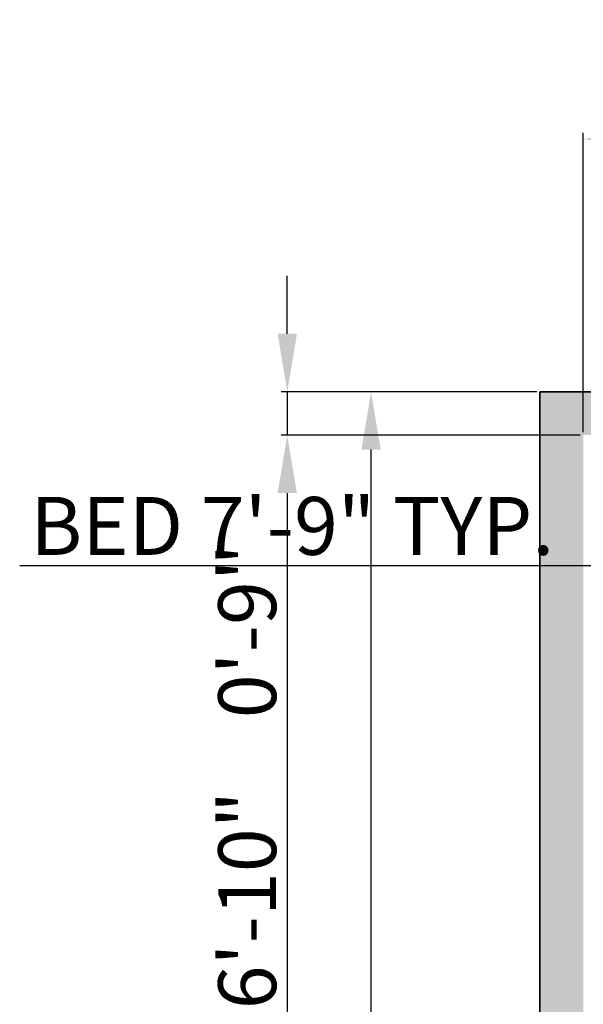
# Model space of a CAD drawing. Units: inches. Extents: x 2083 to 3317, y 1141 to 2115.
# Tile 94 of 256: x 2119 to 2236, y 1894 to 2098. Entities that reach past the tile are written whole.
import ezdxf

# ---------------------------------------------------------------- set-up
doc = ezdxf.new("R2010")
doc.units = ezdxf.units.IN
doc.layers.add('A-ANNO-DIMS', color=2, linetype='Continuous', lineweight=18)
doc.layers.add('A-WALL', color=7, linetype='Continuous', lineweight=35)
doc.layers.add('A-WALL-PATT', color=251, linetype='Continuous', lineweight=13, true_color=0x636466)
doc.styles.get("Standard").update_dxf_attribs({"font": 'arial.ttf'})
doc.dimstyles.new('ISO-25', dxfattribs={"dimtxt": 12, "dimasz": 12, "dimexe": 1.25, "dimexo": 0.625, "dimtad": 1, "dimlunit": 3, "dimtxsty": 'Standard', "dimcen": 2.5, "dimadec": 0, "dimazin": 0, "dimtfac": 1, "dimtmove": 0, "dimatfit": 3, "dimfxl": 1, "dimarcsym": 0})

# ---------------------------------------------------------------- blocks, each defined once
blk = doc.blocks.new('*D14')
at = {"layer": 'A-ANNO-DIMS', "color": 0, "lineweight": -2, "transparency": 16777216}
for p, q in [((2226.33, 2020.76), (2190.73, 2020.76)), ((2191.98, 1714.76), (2191.98, 2008.76)), ((2226.33, 1702.76), (2190.73, 1702.76))]:
    blk.add_line(p, q, dxfattribs=at)
at = {"layer": 'A-ANNO-DIMS', "color": 0, "transparency": 16777216}
for points in [[(2189.98, 2008.76), (2193.98, 2008.76), (2191.98, 2020.76)], [(2189.98, 1714.76), (2193.98, 1714.76), (2191.98, 1702.76)]]:
    blk.add_solid(points, dxfattribs=at)
at = {"layer": 'Defpoints', "color": 0, "transparency": 16777216}
for p in [(2191.98, 2020.76), (2226.96, 2020.76), (2226.96, 1702.76)]:
    blk.add_point(p, dxfattribs=at)
at = {"layer": 'A-ANNO-DIMS', "color": 0, "transparency": 16777216, "insert": (2185.22, 1861.76), "char_height": 12, "attachment_point": 5, "rotation": 90}
blk.add_mtext('26\'-6"', dxfattribs=at)
blk = doc.blocks.new('*D20')
at = {"layer": 'A-ANNO-DIMS', "color": 0, "lineweight": -2, "transparency": 16777216}
for p, q in [((2244.15, 1971.32), (2244.15, 1985.9)), ((2337.22, 1971.32), (2337.22, 1985.9)), ((2244.15, 1984.65), (2119.16, 1984.65)), ((2325.22, 1984.65), (2256.15, 1984.65))]:
    blk.add_line(p, q, dxfattribs=at)
at = {"layer": 'A-ANNO-DIMS', "color": 0, "transparency": 16777216}
for points in [[(2256.15, 1986.65), (2256.15, 1982.65), (2244.15, 1984.65)], [(2325.22, 1986.65), (2325.22, 1982.65), (2337.22, 1984.65)]]:
    blk.add_solid(points, dxfattribs=at)
at = {"layer": 'Defpoints', "color": 0, "transparency": 16777216}
for p in [(2244.15, 1984.65), (2244.15, 1970.69), (2337.22, 1970.69)]:
    blk.add_point(p, dxfattribs=at)
at = {"layer": 'A-ANNO-DIMS', "color": 0, "transparency": 16777216, "insert": (2175.65, 1991.4), "char_height": 12, "attachment_point": 5}
blk.add_mtext('BED 7\'-9" TYP.', dxfattribs=at)
blk = doc.blocks.new('*D36')
at = {"layer": 'A-ANNO-DIMS', "color": 0, "lineweight": -2, "transparency": 16777216}
for p, q in [((2235.96, 2012.39), (2235.96, 2074.36)), ((2247.96, 2073.11), (2459.46, 2073.11)), ((2471.46, 2012.39), (2471.46, 2074.36))]:
    blk.add_line(p, q, dxfattribs=at)
at = {"layer": 'A-ANNO-DIMS', "color": 0, "transparency": 16777216}
for points in [[(2247.96, 2075.11), (2247.96, 2071.11), (2235.96, 2073.11)], [(2459.46, 2075.11), (2459.46, 2071.11), (2471.46, 2073.11)]]:
    blk.add_solid(points, dxfattribs=at)
at = {"layer": 'Defpoints', "color": 0, "transparency": 16777216}
for p in [(2471.46, 2073.11), (2235.96, 2011.76), (2471.46, 2011.76)]:
    blk.add_point(p, dxfattribs=at)
at = {"layer": 'A-ANNO-DIMS', "color": 0, "transparency": 16777216, "insert": (2353.71, 2079.94), "char_height": 12, "attachment_point": 5}
blk.add_mtext('19\'-7 1/2"', dxfattribs=at)
blk = doc.blocks.new('*D39')
at = {"layer": 'A-ANNO-DIMS', "color": 0, "lineweight": -2, "transparency": 16777216}
for p, q in [((2235.33, 2011.76), (2173.36, 2011.76)), ((2174.61, 1999.76), (2174.61, 1822.01)), ((2235.33, 1810.01), (2173.36, 1810.01))]:
    blk.add_line(p, q, dxfattribs=at)
at = {"layer": 'A-ANNO-DIMS', "color": 0, "transparency": 16777216}
for points in [[(2172.61, 1999.76), (2176.61, 1999.76), (2174.61, 2011.76)], [(2172.61, 1822.01), (2176.61, 1822.01), (2174.61, 1810.01)]]:
    blk.add_solid(points, dxfattribs=at)
at = {"layer": 'Defpoints', "color": 0, "transparency": 16777216}
for p in [(2235.96, 2011.76), (2174.61, 1810.01), (2235.96, 1810.01)]:
    blk.add_point(p, dxfattribs=at)
at = {"layer": 'A-ANNO-DIMS', "color": 0, "transparency": 16777216, "insert": (2167.86, 1910.89), "char_height": 12, "attachment_point": 5, "rotation": 90}
blk.add_mtext('16\'-10"', dxfattribs=at)
blk = doc.blocks.new('*D49')
at = {"layer": 'A-ANNO-DIMS', "color": 0, "lineweight": -2, "transparency": 16777216}
for p, q in [((2174.61, 2032.76), (2174.61, 2044.76)), ((2226.33, 2020.76), (2173.36, 2020.76)), ((2174.61, 2020.76), (2174.61, 2011.76)), ((2235.33, 2011.76), (2173.36, 2011.76)), ((2174.61, 1999.76), (2174.61, 1954.61))]:
    blk.add_line(p, q, dxfattribs=at)
at = {"layer": 'A-ANNO-DIMS', "color": 0, "transparency": 16777216}
for points in [[(2172.61, 2032.76), (2176.61, 2032.76), (2174.61, 2020.76)], [(2172.61, 1999.76), (2176.61, 1999.76), (2174.61, 2011.76)]]:
    blk.add_solid(points, dxfattribs=at)
at = {"layer": 'Defpoints', "color": 0, "transparency": 16777216}
for p in [(2226.96, 2020.76), (2174.61, 2011.76), (2235.96, 2011.76)]:
    blk.add_point(p, dxfattribs=at)
at = {"layer": 'A-ANNO-DIMS', "color": 0, "transparency": 16777216, "insert": (2167.86, 1971.19), "char_height": 12, "attachment_point": 5, "rotation": 90}
blk.add_mtext('0\'-9"', dxfattribs=at)

msp = doc.modelspace()

# ---------------------------------------------------------------- hatches: boundary and pattern name
at = {"layer": 'A-WALL-PATT'}
h = msp.add_hatch(color=256, dxfattribs=at)
h.dxf.hatch_style = 1
h.paths.add_polyline_path([(3126.96, 2020.761), (2748.96, 2020.761), (2604.96, 2020.761), (2226.96, 2020.761), (2226.96, 1702.761), (2466.96, 1702.761), (2466.96, 1582.761), (2418.96, 1582.761), (2418.96, 1477.761), (2226.96, 1477.761), (2226.96, 1263.261), (2544.96, 1263.261), (2544.96, 1411.761), (2604.96, 1411.761), (2685.96, 1411.761), (2685.96, 1420.761), (2604.96, 1420.761), (2604.96, 1573.761), (2604.96, 1702.761), (2604.96, 2011.761), (2748.96, 2011.761), (2748.96, 1702.761), (2862.96, 1702.761), (2862.96, 1621.761), (2871.96, 1621.761), (2871.96, 1702.761), (2883.96, 1702.761), (2883.96, 1706.939, -0.0264593), (2883.96, 1711.761), (2757.96, 1711.761), (2757.96, 1807.761), (2787.96, 1807.761), (2787.96, 1812.261), (2757.96, 1812.261), (2757.96, 2011.761), (2877.96, 2011.761), (2877.96, 1812.261), (2847.96, 1812.261), (2847.96, 1807.761), (2889.836, 1807.761), (2889.836, 1812.261), (2882.46, 1812.261), (2882.46, 2011.761), (3117.96, 2011.761), (3117.96, 1812.261), (2937.836, 1812.261), (2937.836, 1807.761), (2995.71, 1807.761), (2995.71, 1796.118), (3000.21, 1796.118), (3000.21, 1807.761), (3117.96, 1807.761), (3117.96, 1711.761), (3000.21, 1711.761), (3000.21, 1760.118), (2998.573, 1760.118, -0.020711), (2995.71, 1760.118), (2995.71, 1711.761), (2931.96, 1711.761), (2931.96, 1702.761), (3126.96, 1702.761)])
h.paths.add_polyline_path([(2471.46, 2011.761), (2471.46, 1810.011), (2462.717, 1810.011), (2462.717, 1805.511), (2505.96, 1805.511), (2505.96, 1810.011), (2475.96, 1810.011), (2475.96, 2011.761), (2595.96, 2011.761), (2595.96, 1810.011), (2565.96, 1810.011), (2565.96, 1805.511), (2595.96, 1805.511), (2595.96, 1711.761), (2235.96, 1711.761), (2235.96, 1805.511), (2353.71, 1805.511), (2353.71, 1796.054), (2358.21, 1796.054), (2358.21, 1805.511), (2414.717, 1805.511), (2414.717, 1810.011), (2235.96, 1810.011), (2235.96, 2011.761)], flags=16)
h.paths.add_polyline_path([(2270.205, 1994.61), (2270.205, 1970.61), (2246.205, 1970.61), (2246.205, 1994.61)], flags=0)
edge = h.paths.add_edge_path(flags=0)
edge.add_ellipse((2332.027, 1899.798), major_axis=(-3.043, 3.043), ratio=0.1682525, start_angle=-161.33217, end_angle=-156.30711, ccw=False)
edge.add_ellipse((2333.082, 1898.744), major_axis=(-1.055, 1.055), ratio=0.4535321, start_angle=-123.37102, end_angle=-94.15911)
edge = h.paths.add_edge_path(flags=0)
edge.add_ellipse((2332.027, 1968.876), major_axis=(3.043, 3.043), ratio=0.1682525, start_angle=18.66783, end_angle=23.69289)
edge.add_spline(control_points=[(2332.926, 1970.691), (2332.227, 1970.336), (2330.894, 1969.659), (2328.413, 1970.932), (2327.204, 1967.749), (2324.71, 1969.956), (2322.533, 1967.012), (2320.013, 1971.296), (2317.68, 1968.158), (2316.041, 1967.102), (2315.427, 1966.81)], knot_values=[0, 0, 0, 0, 2.2670587, 4.3245589, 6.6855835, 8.8786411, 11.121502, 14.300359, 17.7552837, 19.732645, 19.732645, 19.732645, 19.732645], degree=3, periodic=0)
edge.add_ellipse((2332.027, 1968.876), major_axis=(3.043, 3.043), ratio=0.1682525, start_angle=18.66783, end_angle=23.69289, ccw=False)
edge.add_ellipse((2333.082, 1969.931), major_axis=(1.055, 1.055), ratio=0.4535321, start_angle=56.62898, end_angle=85.84089, ccw=False)
edge = h.paths.add_edge_path(flags=0)
edge.add_spline(control_points=[(2296.428, 1967.988), (2293.628, 1965.336), (2287.704, 1959.727), (2299.744, 1949.996), (2294.533, 1935.669), (2290.573, 1920.604), (2293.394, 1909.974), (2296.185, 1904.967)], knot_values=[0.0991853, 0.0991853, 0.0991853, 0.0991853, 0.3453009, 0.6198217, 0.9826526, 1.3860932, 1.8105546, 1.8105546, 1.8105546, 1.8105546], degree=3, periodic=0)
edge.add_spline(control_points=[(2296.185, 1904.967), (2297.384, 1902.619), (2298.001, 1901.949), (2298.553, 1901.468)], knot_values=[0.0062457, 0.0062457, 0.0062457, 0.0062457, 0.0554759, 0.0554759, 0.0554759, 0.0554759], degree=3, periodic=0)
edge.add_spline(control_points=[(2298.553, 1901.468), (2297.259, 1900.923), (2295.225, 1900.232), (2293.06, 1900.614), (2292.101, 1900.788), (2292.09, 1900.791)], knot_values=[0.3128349, 0.3128349, 0.3128349, 0.3128349, 0.4017797, 0.4749867, 0.4759027, 0.4759027, 0.4759027, 0.4759027], degree=3, periodic=0)
edge.add_arc((2292.794, 1904.664), 3.937, 215.4209, 259.69818, ccw=False)
edge.add_spline(control_points=[(2289.585, 1902.382), (2289.477, 1902.535), (2289.368, 1902.688), (2289.261, 1902.841)], knot_values=[0.1028719, 0.1028719, 0.1028719, 0.1028719, 0.1168958, 0.1168958, 0.1168958, 0.1168958], degree=3, periodic=0)
edge.add_spline(control_points=[(2289.261, 1902.841), (2288.687, 1902.55), (2287.64, 1902.02), (2285.881, 1901.874), (2283.853, 1901.504), (2281.72, 1899.711), (2278.467, 1899.493), (2276.157, 1901.883), (2272.259, 1899.804), (2267.778, 1901.843), (2262.244, 1900.184), (2257.415, 1901.782), (2254.318, 1900.726), (2253.178, 1900.337)], knot_values=[0, 0, 0, 0, 1.9079767, 3.4771759, 5.261074, 7.9728515, 11.6802485, 13.7179214, 16.9395917, 22.789562, 27.5025027, 33.5952153, 37.1456181, 37.1456181, 37.1456181, 37.1456181], degree=3, periodic=0)
edge.add_line((2253.178, 1900.337), (2250.244, 1902.841))
edge.add_line((2250.244, 1902.841), (2250.244, 1965.833))
edge.add_line((2250.244, 1965.833), (2253.178, 1968.337))
edge.add_spline(control_points=[(2253.178, 1968.337), (2254.318, 1967.948), (2257.415, 1966.892), (2262.244, 1968.49), (2267.778, 1966.831), (2271.527, 1968.537), (2273.876, 1967.828), (2274.207, 1967.728)], knot_values=[0, 0, 0, 0, 0.0901802, 0.2449351, 0.3646438, 0.5132331, 0.5378548, 0.5378548, 0.5378548, 0.5378548], degree=3, periodic=0)
edge.add_arc((2274.353, 1963.793), 3.937, 72.05113, 92.12795, ccw=False)
edge.add_arc((2281.297, 1985.23), 18.596, 252.05113, 288.56572)
edge.add_arc((2292.317, 1956.029), 12.646, 71.02679, 113.77822, ccw=False)
edge = h.paths.add_edge_path(flags=0)
edge.add_spline(control_points=[(2274.899, 1951.856), (2275.066, 1951.617), (2275.233, 1951.377), (2275.398, 1951.136)], knot_values=[1.4099157, 1.4099157, 1.4099157, 1.4099157, 1.4315903, 1.4315903, 1.4315903, 1.4315903], degree=3, periodic=0)
edge.add_spline(control_points=[(2275.398, 1951.136), (2275.792, 1950.562), (2276.179, 1949.984), (2276.546, 1949.397)], knot_values=[1.3582378, 1.3582378, 1.3582378, 1.3582378, 1.4099157, 1.4099157, 1.4099157, 1.4099157], degree=3, periodic=0)
edge.add_line((2276.546, 1949.397), (2277.437, 1947.862))
edge.add_spline(control_points=[(2277.437, 1947.862), (2276.304, 1945.673), (2274.64, 1942.427), (2274.632, 1938.094), (2272.799, 1930.852), (2274.356, 1943.897), (2275.948, 1947.923), (2276.546, 1949.397)], knot_values=[0.0056315, 0.0056315, 0.0056315, 0.0056315, 0.1860139, 0.2660015, 0.3570872, 0.5963902, 0.7397317, 0.7397317, 0.7397317, 0.7397317], degree=3, periodic=0)
edge.add_spline(control_points=[(2276.546, 1949.397), (2276.179, 1949.984), (2275.792, 1950.562), (2275.398, 1951.136)], knot_values=[1.3582378, 1.3582378, 1.3582378, 1.3582378, 1.4099157, 1.4099157, 1.4099157, 1.4099157], degree=3, periodic=0)
edge.add_spline(control_points=[(2275.398, 1951.136), (2274.943, 1950.08), (2274.208, 1948.025), (2273.935, 1944.851), (2272.469, 1937.627), (2273.466, 1945.696), (2274.701, 1951.059), (2274.899, 1951.856)], knot_values=[0.1043639, 0.1043639, 0.1043639, 0.1043639, 0.1896363, 0.2696239, 0.3607096, 0.6000126, 0.6446217, 0.6446217, 0.6446217, 0.6446217], degree=3, periodic=0)
h.paths.add_polyline_path([(2269.168, 1963.128, -0.3575267), (2268.171, 1960.976, -0.0925607), (2268.171, 1939.436, -0.3575267), (2269.168, 1937.285, -0.3575267), (2267.016, 1938.282, -0.1647847), (2254.686, 1938.282, -0.3575267), (2252.534, 1937.285, -0.3575267), (2253.531, 1939.436, -0.0925607), (2253.531, 1960.976, -0.3575267), (2252.534, 1963.128, -0.3575267), (2254.686, 1962.131, -0.1647847), (2267.016, 1962.131, -0.3575267)], flags=0)
h.paths.add_polyline_path([(2248.874, 1967.802), (2248.874, 1957.028), (2249.458, 1957.028), (2249.458, 1911.647), (2248.874, 1911.647), (2248.874, 1900.873), (2246.512, 1900.873, 0.1973271), (2244.15, 1902.457), (2244.15, 1966.218, 0.1973271), (2246.512, 1967.802)], flags=0)
h.paths.add_polyline_path([(2269.168, 1931.389, -0.3575267), (2268.171, 1929.238, -0.0925607), (2268.171, 1907.698, -0.3575267), (2269.168, 1905.547, -0.3575267), (2267.016, 1906.544, -0.1647847), (2254.686, 1906.544, -0.3575267), (2252.534, 1905.547, -0.3575267), (2253.531, 1907.698, -0.0925607), (2253.531, 1929.238, -0.3575267), (2252.534, 1931.389, -0.3575267), (2254.686, 1930.392, -0.1647847), (2267.016, 1930.392, -0.3575267)], flags=0)
edge = h.paths.add_edge_path(flags=0)
edge.add_spline(control_points=[(2276.197, 1906.724), (2276.168, 1909.029), (2276.114, 1913.372), (2270.598, 1924.925), (2273.905, 1919.013), (2275.922, 1916.262), (2275.475, 1912.402), (2277.258, 1910.381), (2276.696, 1908.225), (2276.646, 1906.813), (2276.618, 1906.008)], knot_values=[0, 0, 0, 0, 8.6102597, 16.2212739, 18.8430575, 23.8048978, 27.4408283, 29.3561016, 31.2034776, 33.6506866, 33.6506866, 33.6506866, 33.6506866], degree=3, periodic=0)
edge.add_spline(control_points=[(2276.618, 1906.008), (2276.623, 1905.624), (2276.498, 1904.629), (2275.442, 1903.855), (2274.937, 1903.08), (2274.859, 1902.841)], knot_values=[0.1564884, 0.1564884, 0.1564884, 0.1564884, 0.1843975, 0.2313765, 0.2505985, 0.2505985, 0.2505985, 0.2505985], degree=3, periodic=0)
edge.add_line((2274.859, 1902.841), (2276.506, 1902.841))
edge.add_spline(control_points=[(2276.506, 1902.841), (2276.788, 1903.085), (2277.665, 1904.125), (2278.25, 1904.341), (2277.654, 1908.527), (2278.156, 1906.228), (2278.1, 1905.286), (2278.847, 1904.069), (2277.857, 1903.415), (2277.874, 1902.991), (2277.904, 1902.841)], knot_values=[0.0595743, 0.0595743, 0.0595743, 0.0595743, 0.0807529, 0.1037415, 0.1697201, 0.1760361, 0.2071372, 0.2404744, 0.2623409, 0.2736605, 0.2736605, 0.2736605, 0.2736605], degree=3, periodic=0)
edge.add_line((2277.904, 1902.841), (2280.03, 1902.841))
edge.add_spline(control_points=[(2280.03, 1902.841), (2279.888, 1903.088), (2279.499, 1903.982), (2280.152, 1905.939), (2278.104, 1909.658), (2279.762, 1907.185), (2280.328, 1904.875), (2280.485, 1903.49), (2281.463, 1903.249), (2281.758, 1902.936), (2281.834, 1902.841)], knot_values=[0.013856, 0.013856, 0.013856, 0.013856, 0.0348738, 0.0888667, 0.1078792, 0.1267378, 0.158714, 0.1937575, 0.2174868, 0.2267221, 0.2267221, 0.2267221, 0.2267221], degree=3, periodic=0)
edge.add_spline(control_points=[(2281.834, 1902.841), (2281.788, 1902.827), (2281.647, 1902.783), (2281.396, 1902.859), (2281.088, 1902.985), (2280.721, 1903.061), (2280.333, 1903.026), (2280.125, 1902.899), (2280.03, 1902.841)], knot_values=[0, 0, 0, 0, 0.1441304, 0.435517, 0.7492759, 1.1530457, 1.5483707, 1.878348, 1.878348, 1.878348, 1.878348], degree=3, periodic=0)
edge.add_line((2280.03, 1902.841), (2277.904, 1902.841))
edge.add_spline(control_points=[(2277.904, 1902.841), (2277.893, 1902.796), (2277.865, 1902.68), (2277.607, 1902.687), (2277.274, 1902.801), (2276.838, 1902.62), (2276.584, 1902.789), (2276.506, 1902.841)], knot_values=[0, 0, 0, 0, 0.1271885, 0.3261988, 0.6280094, 1.2435704, 1.5153306, 1.5153306, 1.5153306, 1.5153306], degree=3, periodic=0)
edge.add_line((2276.506, 1902.841), (2274.859, 1902.841))
edge.add_spline(control_points=[(2274.859, 1902.841), (2274.814, 1902.899), (2274.725, 1903.013), (2274.493, 1903.119), (2274.244, 1902.961), (2273.937, 1903.185), (2273.614, 1902.983), (2273.408, 1902.883), (2273.322, 1902.841)], knot_values=[0, 0, 0, 0, 0.2184302, 0.4369566, 0.6879766, 0.9903786, 1.3983955, 1.6918498, 1.6918498, 1.6918498, 1.6918498], degree=3, periodic=0)
edge.add_spline(control_points=[(2273.322, 1902.841), (2273.617, 1903.446), (2274.274, 1904.538), (2276.027, 1904.574), (2276.207, 1906.584), (2276.197, 1906.724)], knot_values=[0.0122268, 0.0122268, 0.0122268, 0.0122268, 0.0594721, 0.1062177, 0.134458, 0.134458, 0.134458, 0.134458], degree=3, periodic=0)
h.paths.add_polyline_path([(2270.776, 1897.79), (2270.776, 1873.79), (2246.776, 1873.79), (2246.776, 1897.79)], flags=0)
h.paths.add_polyline_path([(2353.71, 1760.005), (2353.71, 1760.054), (2358.21, 1760.054, -0.033729)], flags=0)
h.paths.add_polyline_path([(2321.819, 1737.529), (2341.995, 1737.529, -0.4142136), (2343.203, 1736.321), (2343.203, 1721.021, -0.4142136), (2341.995, 1719.813), (2321.819, 1719.813, -0.4142136), (2320.611, 1721.021), (2320.611, 1736.321, -0.4142136)], flags=0)
h.paths.add_polyline_path([(2324.235, 1736.321), (2339.579, 1736.321, -0.4142136), (2341.995, 1733.905), (2341.995, 1725.45, -0.4142136), (2339.579, 1723.034), (2333.681, 1723.034), (2333.845, 1722.045, -0.8706461), (2335.425, 1721.826, -0.767327), (2333.923, 1721.423), (2331.291, 1721.423, -0.767327), (2329.788, 1721.826, -0.8706461), (2331.368, 1722.045), (2331.533, 1723.034), (2324.235, 1723.034, -0.4142136), (2321.819, 1725.45), (2321.819, 1733.905, -0.4142136)], flags=0)
h.paths.add_polyline_path([(2570.484, 1928.615), (2589.684, 1928.615), (2590.169, 1928.615), (2590.169, 1904.993), (2570.484, 1904.993)], flags=0)
h.paths.add_polyline_path([(2574.447, 1927.264, -1), (2572.829, 1927.264, -1)], flags=0)
h.paths.add_polyline_path([(2573.09, 1926.941), (2573.925, 1927.776), (2574.148, 1927.553), (2573.313, 1926.718)], flags=0)
h.paths.add_polyline_path([(2578.779, 1919.73, -1), (2571.592, 1919.73, -1)], flags=0)
h.paths.add_polyline_path([(2578.385, 1919.73, -1), (2571.985, 1919.73, -1)], flags=0)
h.paths.add_polyline_path([(2331.596, 1729.476, -1), (2333.618, 1729.476, -1)], flags=0)
h.paths.add_polyline_path([(2578.034, 1927.264, -1), (2576.416, 1927.264, -1)], flags=0)
h.paths.add_polyline_path([(2576.689, 1927.531), (2576.912, 1927.754), (2577.747, 1926.919), (2577.524, 1926.696)], flags=0)
h.paths.add_polyline_path([(2578.139, 1909.86, -1), (2572.232, 1909.86, -1)], flags=0)
h.paths.add_polyline_path([(2577.745, 1909.86, -1), (2572.625, 1909.86, -1)], flags=0)
h.paths.add_polyline_path([(2583.798, 1927.264, -1), (2582.179, 1927.264, -1)], flags=0)
h.paths.add_polyline_path([(2582.719, 1927.754), (2583.554, 1926.919), (2583.331, 1926.696), (2582.496, 1927.531)], flags=0)
h.paths.add_polyline_path([(2582.496, 1927.531), (2582.719, 1927.754), (2583.554, 1926.919), (2583.331, 1926.696)], flags=0)
h.paths.add_polyline_path([(2587.739, 1920.53, -1), (2581.832, 1920.53, -1)], flags=0)
h.paths.add_polyline_path([(2587.345, 1920.53, -1), (2582.225, 1920.53, -1)], flags=0)
h.paths.add_polyline_path([(2587.385, 1927.264, -1), (2585.766, 1927.264, -1)], flags=0)
h.paths.add_polyline_path([(2586.082, 1926.98), (2586.917, 1927.815), (2587.14, 1927.593), (2586.305, 1926.758)], flags=0)
h.paths.add_polyline_path([(2588.379, 1910.66, -1), (2581.192, 1910.66, -1)], flags=0)
h.paths.add_polyline_path([(2587.985, 1910.66, -1), (2581.585, 1910.66, -1)], flags=0)
h.paths.add_polyline_path([(2417.168, 1729.478), (2437.344, 1729.478, -0.4142136), (2438.552, 1728.27), (2438.552, 1712.969, -0.4142136), (2437.344, 1711.761), (2417.168, 1711.761, -0.4142136), (2415.96, 1712.969), (2415.96, 1728.27, -0.4142136)], flags=0)
h.paths.add_polyline_path([(2419.584, 1728.27), (2434.928, 1728.27, -0.4142136), (2437.344, 1725.854), (2437.344, 1717.398, -0.4142136), (2434.928, 1714.983), (2429.029, 1714.983), (2429.194, 1713.994, -0.8706461), (2430.774, 1713.775, -0.767327), (2429.271, 1713.372), (2426.64, 1713.372, -0.767327), (2425.137, 1713.775, -0.8706461), (2426.717, 1713.994), (2426.882, 1714.983), (2419.584, 1714.983, -0.4142136), (2417.168, 1717.398), (2417.168, 1725.854, -0.4142136)], flags=0)
h.paths.add_polyline_path([(2419.584, 1728.27), (2434.928, 1728.27, -0.4142136), (2437.344, 1725.854), (2437.344, 1717.398, -0.4142136), (2434.928, 1714.983), (2429.029, 1714.983), (2428.358, 1719.009), (2427.553, 1719.009), (2426.882, 1714.983), (2419.584, 1714.983, -0.4142136), (2417.168, 1717.398), (2417.168, 1725.854, -0.4142136)], flags=0)
h.paths.add_polyline_path([(2426.944, 1721.425, -1), (2428.967, 1721.425, -1)], flags=0)
h.paths.add_polyline_path([(2475.96, 1702.761), (2595.96, 1702.761), (2595.96, 1582.761), (2475.96, 1582.761)], flags=16)
h.paths.add_polyline_path([(2427.96, 1573.761), (2595.96, 1573.761), (2595.96, 1468.761), (2595.96, 1420.761), (2384.46, 1420.761), (2384.46, 1468.761), (2427.96, 1468.761)], flags=16)
h.paths.add_polyline_path([(2379.96, 1468.761), (2379.96, 1420.761), (2235.96, 1420.761), (2235.96, 1468.761)], flags=16)
h.paths.add_polyline_path([(2317.816, 1466.696), (2337.992, 1466.696, -0.4142136), (2339.2, 1465.488), (2339.2, 1450.187, -0.4142136), (2337.992, 1448.979), (2317.816, 1448.979, -0.4142136), (2316.608, 1450.187), (2316.608, 1465.488, -0.4142136)], flags=0)
h.paths.add_polyline_path([(2320.232, 1465.488), (2335.576, 1465.488, -0.4142136), (2337.992, 1463.072), (2337.992, 1454.616, -0.4142136), (2335.576, 1452.2), (2329.677, 1452.2), (2329.842, 1451.212, -0.8706461), (2331.422, 1450.992, -0.767327), (2329.92, 1450.59), (2327.288, 1450.59, -0.767327), (2325.785, 1450.992, -0.8706461), (2327.365, 1451.212), (2327.53, 1452.2), (2320.232, 1452.2, -0.4142136), (2317.816, 1454.616), (2317.816, 1463.072, -0.4142136)], flags=0)
h.paths.add_polyline_path([(2320.232, 1465.488), (2335.576, 1465.488, -0.4142136), (2337.992, 1463.072), (2337.992, 1454.616, -0.4142136), (2335.576, 1452.2), (2329.677, 1452.2), (2329.006, 1456.227), (2328.201, 1456.227), (2327.53, 1452.2), (2320.232, 1452.2, -0.4142136), (2317.816, 1454.616), (2317.816, 1463.072, -0.4142136)], flags=0)
h.paths.add_polyline_path([(2327.593, 1458.643, -1), (2329.615, 1458.643, -1)], flags=0)
h.paths.add_polyline_path([(2244.412, 1433.34), (2241.921, 1433.34, -0.4142136), (2240.018, 1435.244), (2240.018, 1440.953, -0.4142105), (2241.921, 1442.856), (2244.412, 1442.856, -1.9764724)], flags=0)
h.paths.add_polyline_path([(2245.357, 1434.398, -0.4142136), (2245.357, 1441.799, -2.1440985)], flags=0)
h.paths.add_polyline_path([(2535.96, 1416.261), (2535.96, 1272.261), (2235.96, 1272.261), (2235.96, 1416.261)], flags=16)
h.paths.add_polyline_path([(2260.12, 1384.293), (2260.12, 1362.039), (2237.865, 1362.039), (2237.865, 1384.293)], flags=0)
edge = h.paths.add_edge_path(flags=0)
edge.add_line((2318.252, 1362.093), (2318.146, 1362.001))
edge.add_ellipse((2317.445, 1360.431), major_axis=(2.822, 2.822), ratio=0.1682525, start_angle=18.66783, end_angle=20.94813, ccw=False)
edge.add_ellipse((2318.423, 1361.409), major_axis=(0.978, 0.978), ratio=0.4535321, start_angle=56.62898, end_angle=70.2262, ccw=False)
edge = h.paths.add_edge_path(flags=0)
edge.add_line((2319.107, 1295.571), (2319.015, 1295.677))
edge.add_ellipse((2317.445, 1296.378), major_axis=(-2.822, 2.822), ratio=0.1682525, start_angle=-161.33217, end_angle=-159.05187, ccw=False)
edge.add_ellipse((2318.423, 1295.4), major_axis=(-0.978, 0.978), ratio=0.4535321, start_angle=-123.37102, end_angle=-109.7738)
edge = h.paths.add_edge_path(flags=0)
edge.add_spline(control_points=[(2284.21, 1301.17), (2284.581, 1300.445), (2284.891, 1299.892), (2285.16, 1299.461)], knot_values=[0.0390658, 0.0390658, 0.0390658, 0.0390658, 0.0554759, 0.0554759, 0.0554759, 0.0554759], degree=3, periodic=0)
edge.add_line((2285.16, 1299.461), (2284.21, 1301.17))
edge = h.paths.add_edge_path(flags=0)
edge.add_line((2280.412, 1297.298), (2283.37, 1297.036))
edge.add_line((2283.37, 1297.036), (2286.406, 1297.926))
edge.add_spline(control_points=[(2286.406, 1297.926), (2285.305, 1297.463), (2284.345, 1297.129), (2283.37, 1297.036)], knot_values=[0.3943688, 0.3943688, 0.3943688, 0.3943688, 0.4759027, 0.4759027, 0.4759027, 0.4759027], degree=3, periodic=0)
edge.add_spline(control_points=[(2283.37, 1297.036), (2283.281, 1297.028), (2282.316, 1296.957), (2281.313, 1297.134), (2280.423, 1297.296), (2280.412, 1297.298)], knot_values=[0.3128349, 0.3128349, 0.3128349, 0.3128349, 0.3202458, 0.3934528, 0.3943688, 0.3943688, 0.3943688, 0.3943688], degree=3, periodic=0)
edge = h.paths.add_edge_path(flags=0)
edge.add_line((2284.436, 1359.607), (2280.446, 1355.328))
edge.add_line((2280.446, 1355.328), (2279.58, 1351.018))
edge.add_line((2279.58, 1351.018), (2282.413, 1346.58))
edge.add_spline(control_points=[(2282.413, 1346.58), (2283.153, 1345.589), (2284.253, 1344.029), (2284.801, 1342.387), (2284.935, 1341.806)], knot_values=[1.2400982, 1.2400982, 1.2400982, 1.2400982, 1.3328922, 1.3827123, 1.3827123, 1.3827123, 1.3827123], degree=3, periodic=0)
edge.add_spline(control_points=[(2284.935, 1341.806), (2285.319, 1340.141), (2285.233, 1338.409), (2284.91, 1336.654)], knot_values=[1.0974841, 1.0974841, 1.0974841, 1.0974841, 1.2400982, 1.2400982, 1.2400982, 1.2400982], degree=3, periodic=0)
edge.add_spline(control_points=[(2284.91, 1336.654), (2284.587, 1334.899), (2284.027, 1333.12), (2283.463, 1331.361)], knot_values=[0.9548699, 0.9548699, 0.9548699, 0.9548699, 1.0974841, 1.0974841, 1.0974841, 1.0974841], degree=3, periodic=0)
edge.add_line((2283.463, 1331.361), (2281.89, 1326.153))
edge.add_line((2281.89, 1326.153), (2280.756, 1321.056))
edge.add_line((2280.756, 1321.056), (2280.299, 1316.002))
edge.add_line((2280.299, 1316.002), (2280.716, 1310.95))
edge.add_line((2280.716, 1310.95), (2282.028, 1305.972))
edge.add_line((2282.028, 1305.972), (2284.21, 1301.17))
edge.add_spline(control_points=[(2284.21, 1301.17), (2283.341, 1302.73), (2282.612, 1304.336), (2282.028, 1305.972)], knot_values=[0.0991853, 0.0991853, 0.0991853, 0.0991853, 0.2417994, 0.2417994, 0.2417994, 0.2417994], degree=3, periodic=0)
edge.add_spline(control_points=[(2282.028, 1305.972), (2281.444, 1307.608), (2281.005, 1309.273), (2280.716, 1310.95)], knot_values=[0.2417994, 0.2417994, 0.2417994, 0.2417994, 0.3844135, 0.3844135, 0.3844135, 0.3844135], degree=3, periodic=0)
edge.add_spline(control_points=[(2280.716, 1310.95), (2280.433, 1312.588), (2280.289, 1314.277), (2280.299, 1315.962), (2280.299, 1316.002)], knot_values=[0.3844135, 0.3844135, 0.3844135, 0.3844135, 0.5236467, 0.5270276, 0.5270276, 0.5270276, 0.5270276], degree=3, periodic=0)
edge.add_spline(control_points=[(2280.299, 1316.002), (2280.312, 1317.687), (2280.478, 1319.368), (2280.756, 1321.056)], knot_values=[0.5270276, 0.5270276, 0.5270276, 0.5270276, 0.6696417, 0.6696417, 0.6696417, 0.6696417], degree=3, periodic=0)
edge.add_spline(control_points=[(2280.756, 1321.056), (2281.035, 1322.744), (2281.426, 1324.44), (2281.89, 1326.153)], knot_values=[0.6696417, 0.6696417, 0.6696417, 0.6696417, 0.8122558, 0.8122558, 0.8122558, 0.8122558], degree=3, periodic=0)
edge.add_spline(control_points=[(2281.89, 1326.153), (2282.264, 1327.533), (2282.788, 1329.262), (2283.353, 1331.018), (2283.463, 1331.361)], knot_values=[0.8122558, 0.8122558, 0.8122558, 0.8122558, 0.9270873, 0.9548699, 0.9548699, 0.9548699, 0.9548699], degree=3, periodic=0)
edge.add_line((2283.463, 1331.361), (2284.91, 1336.654))
edge.add_line((2284.91, 1336.654), (2284.935, 1341.806))
edge.add_line((2284.935, 1341.806), (2282.413, 1346.58))
edge.add_spline(control_points=[(2282.413, 1346.58), (2281.275, 1348.104), (2280.078, 1349.57), (2279.58, 1351.018)], knot_values=[1.3827123, 1.3827123, 1.3827123, 1.3827123, 1.5253264, 1.5253264, 1.5253264, 1.5253264], degree=3, periodic=0)
edge.add_spline(control_points=[(2279.58, 1351.018), (2279.443, 1351.415), (2279.136, 1352.857), (2279.735, 1354.29), (2280.446, 1355.328)], knot_values=[1.5253264, 1.5253264, 1.5253264, 1.5253264, 1.564439, 1.6679405, 1.6679405, 1.6679405, 1.6679405], degree=3, periodic=0)
edge.add_spline(control_points=[(2280.446, 1355.328), (2281.426, 1356.758), (2282.931, 1358.183), (2284.436, 1359.607)], knot_values=[1.6679405, 1.6679405, 1.6679405, 1.6679405, 1.8105546, 1.8105546, 1.8105546, 1.8105546], degree=3, periodic=0)
edge.add_arc((2280.623, 1348.518), 11.726, 71.02679, 113.77822)
edge.add_arc((2270.405, 1375.595), 17.244, 252.05113, 288.56572, ccw=False)
edge.add_arc((2263.966, 1355.718), 3.651, 72.05113, 92.12795)
edge.add_arc((2263.966, 1355.718), 3.651, 92.12795, 177.98513)
edge.add_spline(control_points=[(2260.318, 1355.846), (2260.26, 1354.221), (2260.551, 1350.187), (2262.999, 1346.766), (2264.473, 1344.649)], knot_values=[1.4315903, 1.4315903, 1.4315903, 1.4315903, 1.5641438, 1.7706953, 1.7706953, 1.7706953, 1.7706953], degree=3, periodic=0)
edge.add_line((2264.473, 1344.649), (2264.936, 1343.983))
edge.add_spline(control_points=[(2263.801, 1340.248), (2263.843, 1340.514), (2264.067, 1341.756), (2264.513, 1343.002), (2264.935, 1343.981)], knot_values=[0.5365702, 0.5365702, 0.5365702, 0.5365702, 0.5593494, 0.6446217, 0.6446217, 0.6446217, 0.6446217], degree=3, periodic=0)
edge.add_spline(control_points=[(2264.935, 1343.981), (2265.118, 1343.715), (2265.299, 1343.448), (2265.477, 1343.179)], knot_values=[1.3840767, 1.3840767, 1.3840767, 1.3840767, 1.4099157, 1.4099157, 1.4099157, 1.4099157], degree=3, periodic=0)
edge.add_spline(control_points=[(2265.477, 1343.179), (2265.655, 1342.911), (2265.829, 1342.641), (2265.999, 1342.369)], knot_values=[1.3582378, 1.3582378, 1.3582378, 1.3582378, 1.3840767, 1.3840767, 1.3840767, 1.3840767], degree=3, periodic=0)
edge.add_line((2265.999, 1342.369), (2266.826, 1340.946))
edge.add_spline(control_points=[(2266.826, 1340.946), (2268.894, 1337.09), (2271.398, 1325.843), (2270.516, 1310.569), (2275.919, 1301.861), (2277.79, 1299.199)], knot_values=[0.1168958, 0.1168958, 0.1168958, 0.1168958, 0.4729873, 1.0509689, 1.3137934, 1.3137934, 1.3137934, 1.3137934], degree=3, periodic=0)
edge.add_spline(control_points=[(2277.79, 1299.199), (2277.839, 1299.128), (2277.889, 1299.057), (2277.94, 1298.987)], knot_values=[0.1098839, 0.1098839, 0.1098839, 0.1098839, 0.1168958, 0.1168958, 0.1168958, 0.1168958], degree=3, periodic=0)
edge.add_line((2277.94, 1298.987), (2277.789, 1299.199))
edge.add_spline(control_points=[(2277.789, 1299.199), (2277.257, 1298.929), (2276.286, 1298.438), (2275.039, 1298.334), (2274.383, 1298.239), (2274.215, 1298.209)], knot_values=[33.1218702, 33.1218702, 33.1218702, 33.1218702, 35.0290557, 36.5982549, 37.1448269, 37.1448269, 37.1448269, 37.1448269], degree=3, periodic=0)
edge.add_line((2274.215, 1298.209), (2273.073, 1297.893))
edge.add_spline(control_points=[(2273.073, 1297.893), (2272.323, 1297.58), (2271.039, 1296.511), (2269.248, 1296.226), (2268.423, 1296.375)], knot_values=[26.5325843, 26.5325843, 26.5325843, 26.5325843, 29.198919, 31.8391012, 31.8391012, 31.8391012, 31.8391012], degree=3, periodic=0)
edge.add_line((2268.423, 1296.375), (2263.879, 1297.458))
edge.add_spline(control_points=[(2263.879, 1297.458), (2263.556, 1297.359), (2261.86, 1296.839), (2260.239, 1297.282), (2258.933, 1297.516)], knot_values=[15.9195506, 15.9195506, 15.9195506, 15.9195506, 16.9395917, 21.2260675, 21.2260675, 21.2260675, 21.2260675], degree=3, periodic=0)
edge.add_line((2258.933, 1297.516), (2254.055, 1297.329))
edge.add_spline(control_points=[(2254.055, 1297.329), (2253.756, 1297.296), (2252.114, 1297.165), (2250.462, 1297.544), (2249.13, 1297.668)], knot_values=[5.3065169, 5.3065169, 5.3065169, 5.3065169, 6.2764352, 10.6130337, 10.6130337, 10.6130337, 10.6130337], degree=3, periodic=0)
edge.add_line((2249.13, 1297.668), (2244.332, 1296.878))
edge.add_line((2244.332, 1296.878), (2241.611, 1299.199))
edge.add_line((2241.611, 1299.199), (2241.611, 1357.609))
edge.add_line((2241.611, 1357.609), (2244.332, 1359.931))
edge.add_line((2244.332, 1359.931), (2252.729, 1359.543))
edge.add_spline(control_points=[(2252.729, 1359.543), (2252.871, 1359.546), (2253.306, 1359.548), (2253.74, 1359.514), (2254.032, 1359.482)], knot_values=[0.233291, 0.233291, 0.233291, 0.233291, 0.2449351, 0.2689274, 0.2689274, 0.2689274, 0.2689274], degree=3, periodic=0)
edge.add_line((2254.032, 1359.482), (2259.587, 1359.416))
edge.add_spline(control_points=[(2259.587, 1359.416), (2260.677, 1359.629), (2262.073, 1359.897), (2263.524, 1359.459), (2263.83, 1359.366)], knot_values=[0.4225164, 0.4225164, 0.4225164, 0.4225164, 0.5132331, 0.5378548, 0.5378548, 0.5378548, 0.5378548], degree=3, periodic=0)
edge.add_arc((2263.966, 1355.718), 3.651, 72.05113, 92.12795, ccw=False)
edge.add_arc((2270.405, 1375.595), 17.244, 252.05113, 288.56572)
edge.add_arc((2280.623, 1348.518), 11.726, 71.02679, 113.77822, ccw=False)
h.paths.add_polyline_path([(2240.341, 1359.435), (2240.341, 1349.444), (2240.882, 1349.444), (2240.882, 1307.365), (2240.341, 1307.365), (2240.341, 1297.374), (2238.15, 1297.374, 0.1973271), (2235.96, 1298.843), (2235.96, 1357.966, 0.1973271), (2238.15, 1359.435)], flags=0)
h.paths.add_polyline_path([(2259.158, 1355.101, -0.3575267), (2258.233, 1353.106, -0.0925607), (2258.233, 1333.133, -0.3575267), (2259.158, 1331.138, -0.3575267), (2257.163, 1332.062, -0.1647847), (2245.729, 1332.062, -0.3575267), (2243.735, 1331.138, -0.3575267), (2244.659, 1333.133, -0.0925607), (2244.659, 1353.106, -0.3575267), (2243.735, 1355.101, -0.3575267), (2245.729, 1354.176, -0.1647847), (2257.163, 1354.176, -0.3575267)], flags=0)
edge = h.paths.add_edge_path(flags=0)
edge.add_line((2265.999, 1342.369), (2266.826, 1340.946))
edge.add_line((2266.826, 1340.946), (2265.308, 1337.814))
edge.add_line((2265.308, 1337.814), (2264.358, 1334.653))
edge.add_line((2264.358, 1334.653), (2264.262, 1333.8))
edge.add_spline(control_points=[(2264.262, 1333.8), (2264.208, 1333.187), (2264.162, 1332.366), (2264.007, 1331.414), (2263.969, 1331.202)], knot_values=[0.4644442, 0.4644442, 0.4644442, 0.4644442, 0.5166905, 0.5316081, 0.5316081, 0.5316081, 0.5316081], degree=3, periodic=0)
edge.add_spline(control_points=[(2263.969, 1331.202), (2263.775, 1330.119), (2263.424, 1328.791), (2263.257, 1328.531), (2263.234, 1328.515)], knot_values=[0.3726816, 0.3726816, 0.3726816, 0.3726816, 0.4488497, 0.4644442, 0.4644442, 0.4644442, 0.4644442], degree=3, periodic=0)
edge.add_spline(control_points=[(2263.234, 1328.515), (2263.096, 1328.42), (2263.131, 1329.301), (2263.275, 1330.616)], knot_values=[0.2809191, 0.2809191, 0.2809191, 0.2809191, 0.3726816, 0.3726816, 0.3726816, 0.3726816], degree=3, periodic=0)
edge.add_spline(control_points=[(2263.275, 1330.616), (2263.419, 1331.93), (2263.672, 1333.677), (2263.97, 1335.315)], knot_values=[0.1891566, 0.1891566, 0.1891566, 0.1891566, 0.2809191, 0.2809191, 0.2809191, 0.2809191], degree=3, periodic=0)
edge.add_spline(control_points=[(2263.97, 1335.315), (2264.1, 1336.032), (2264.419, 1337.622), (2264.755, 1338.864), (2264.947, 1339.491)], knot_values=[0.097394, 0.097394, 0.097394, 0.097394, 0.1375775, 0.1891566, 0.1891566, 0.1891566, 0.1891566], degree=3, periodic=0)
edge.add_spline(control_points=[(2264.947, 1339.491), (2265.29, 1340.606), (2265.644, 1341.494), (2265.999, 1342.369)], knot_values=[0.0056315, 0.0056315, 0.0056315, 0.0056315, 0.097394, 0.097394, 0.097394, 0.097394], degree=3, periodic=0)
h.paths.add_polyline_path([(2259.158, 1325.671, -0.3575267), (2258.233, 1323.676, -0.0925607), (2258.233, 1303.703, -0.3575267), (2259.158, 1301.708, -0.3575267), (2257.163, 1302.633, -0.1647847), (2245.729, 1302.633, -0.3575267), (2243.735, 1301.708, -0.3575267), (2244.659, 1303.703, -0.0925607), (2244.659, 1323.676, -0.3575267), (2243.735, 1325.671, -0.3575267), (2245.729, 1324.747, -0.1647847), (2257.163, 1324.747, -0.3575267)], flags=0)
edge = h.paths.add_edge_path(flags=0)
edge.add_spline(control_points=[(2261.709, 1317.311), (2261.679, 1317.418), (2261.762, 1317.389), (2262.491, 1316.09), (2262.962, 1315.301)], knot_values=[14.9558607, 14.9558607, 14.9558607, 14.9558607, 16.2212739, 18.6948259, 18.6948259, 18.6948259, 18.6948259], degree=3, periodic=0)
edge.add_spline(control_points=[(2262.962, 1315.301), (2262.99, 1315.254), (2263.702, 1314.067), (2264.349, 1313.127), (2264.73, 1312.164)], knot_values=[18.6948259, 18.6948259, 18.6948259, 18.6948259, 18.8430575, 22.433791, 22.433791, 22.433791, 22.433791], degree=3, periodic=0)
edge.add_spline(control_points=[(2264.73, 1312.164), (2264.876, 1311.796), (2265.177, 1310.77), (2265.143, 1309.559), (2265.248, 1308.824)], knot_values=[22.433791, 22.433791, 22.433791, 22.433791, 23.8048978, 26.1727562, 26.1727562, 26.1727562, 26.1727562], degree=3, periodic=0)
edge.add_line((2265.248, 1308.824), (2265.851, 1307.172))
edge.add_spline(control_points=[(2265.851, 1307.172), (2266.065, 1306.822), (2266.384, 1306.332), (2266.424, 1305.781), (2266.42, 1305.611)], knot_values=[28.0625624, 28.0625624, 28.0625624, 28.0625624, 29.3561016, 29.9117214, 29.9117214, 29.9117214, 29.9117214], degree=3, periodic=0)
edge.add_spline(control_points=[(2266.42, 1305.611), (2266.416, 1305.433), (2266.394, 1305.25), (2266.365, 1305.066)], knot_values=[29.9117214, 29.9117214, 29.9117214, 29.9117214, 30.4978371, 30.4978371, 30.4978371, 30.4978371], degree=3, periodic=0)
edge.add_line((2266.365, 1305.066), (2266.066, 1302.136))
edge.add_spline(control_points=[(2266.066, 1302.136), (2266.071, 1301.78), (2265.998, 1301.2), (2265.663, 1300.759), (2265.509, 1300.586)], knot_values=[0.1564884, 0.1564884, 0.1564884, 0.1564884, 0.1843975, 0.2035434, 0.2035434, 0.2035434, 0.2035434], degree=3, periodic=0)
edge.add_line((2265.509, 1300.586), (2264.435, 1299.199))
edge.add_line((2264.435, 1299.199), (2265.962, 1299.199))
edge.add_line((2265.962, 1299.199), (2267.336, 1301.175))
edge.add_line((2267.336, 1301.175), (2267.312, 1301.986))
edge.add_spline(control_points=[(2267.312, 1301.986), (2267.261, 1302.862), (2267.16, 1303.737), (2267.271, 1303.326)], knot_values=[0.1262286, 0.1262286, 0.1262286, 0.1262286, 0.1666174, 0.1666174, 0.1666174, 0.1666174], degree=3, periodic=0)
edge.add_spline(control_points=[(2267.271, 1303.326), (2267.28, 1303.294), (2267.31, 1303.175), (2267.373, 1302.884), (2267.406, 1302.683), (2267.418, 1302.601)], knot_values=[0.1666174, 0.1666174, 0.1666174, 0.1666174, 0.1697201, 0.1760361, 0.1807647, 0.1807647, 0.1807647, 0.1807647], degree=3, periodic=0)
edge.add_spline(control_points=[(2267.744, 1300.988), (2267.688, 1301.151), (2267.481, 1301.657), (2267.484, 1302.145), (2267.418, 1302.601)], knot_values=[0.1807647, 0.1807647, 0.1807647, 0.1807647, 0.1937665, 0.2201389, 0.2201389, 0.2201389, 0.2201389], degree=3, periodic=0)
edge.add_line((2267.418, 1302.601), (2267.744, 1300.988))
edge.add_spline(control_points=[(2267.744, 1300.988), (2267.832, 1300.732), (2267.932, 1300.31), (2267.555, 1299.975), (2267.429, 1299.829)], knot_values=[0.2201389, 0.2201389, 0.2201389, 0.2201389, 0.2404744, 0.2548903, 0.2548903, 0.2548903, 0.2548903], degree=3, periodic=0)
edge.add_line((2267.429, 1299.829), (2267.258, 1299.199))
edge.add_line((2267.258, 1299.199), (2269.23, 1299.199))
edge.add_spline(control_points=[(2269.23, 1299.199), (2269.099, 1299.429), (2268.843, 1300.016), (2269.012, 1300.916), (2268.947, 1301.661)], knot_values=[0.013856, 0.013856, 0.013856, 0.013856, 0.0348738, 0.0670726, 0.0670726, 0.0670726, 0.0670726], degree=3, periodic=0)
edge.add_line((2268.947, 1301.661), (2268.432, 1303.603))
edge.add_spline(control_points=[(2268.432, 1303.603), (2268.176, 1304.192), (2267.596, 1305.251), (2268.041, 1304.623), (2268.251, 1304.282)], knot_values=[0.0901547, 0.0901547, 0.0901547, 0.0901547, 0.1078792, 0.1202891, 0.1202891, 0.1202891, 0.1202891], degree=3, periodic=0)
edge.add_spline(control_points=[(2268.251, 1304.282), (2268.361, 1304.105), (2269.058, 1302.918), (2269.383, 1301.59), (2269.521, 1300.776), (2269.575, 1300.556)], knot_values=[0.1202891, 0.1202891, 0.1202891, 0.1202891, 0.1267378, 0.158714, 0.1735056, 0.1735056, 0.1735056, 0.1735056], degree=3, periodic=0)
edge.add_line((2269.575, 1300.556), (2270.686, 1299.421))
edge.add_spline(control_points=[(2270.686, 1299.421), (2270.767, 1299.357), (2270.838, 1299.281), (2270.903, 1299.199)], knot_values=[0.2181597, 0.2181597, 0.2181597, 0.2181597, 0.2267221, 0.2267221, 0.2267221, 0.2267221], degree=3, periodic=0)
edge.add_line((2270.937, 1299.193), (2270.903, 1299.199))
edge.add_spline(control_points=[(2270.903, 1299.199), (2270.86, 1299.186), (2270.73, 1299.146), (2270.496, 1299.216), (2270.272, 1299.308), (2270.121, 1299.348), (2270.063, 1299.36)], knot_values=[0.939174, 0.939174, 0.939174, 0.939174, 1.0833044, 1.3746911, 1.6884499, 1.878348, 1.878348, 1.878348, 1.878348], degree=3, periodic=0)
edge.add_line((2270.063, 1299.36), (2269.23, 1299.199))
edge.add_line((2269.23, 1299.199), (2267.258, 1299.199))
edge.add_spline(control_points=[(2267.258, 1299.199), (2267.248, 1299.157), (2267.223, 1299.05), (2266.984, 1299.057), (2266.809, 1299.116), (2266.677, 1299.109), (2266.637, 1299.105)], knot_values=[0.7576653, 0.7576653, 0.7576653, 0.7576653, 0.8848538, 1.0838641, 1.3856747, 1.5153306, 1.5153306, 1.5153306, 1.5153306], degree=3, periodic=0)
edge.add_spline(control_points=[(2266.637, 1299.105), (2266.485, 1299.089), (2266.236, 1299.017), (2266.035, 1299.151), (2265.962, 1299.199)], knot_values=[0, 0, 0, 0, 0.4859051, 0.7576653, 0.7576653, 0.7576653, 0.7576653], degree=3, periodic=0)
edge.add_line((2265.962, 1299.199), (2264.435, 1299.199))
edge.add_line((2264.435, 1299.199), (2263.858, 1299.367))
edge.add_spline(control_points=[(2263.858, 1299.367), (2263.819, 1299.371), (2263.78, 1299.386), (2263.74, 1299.402)], knot_values=[0.8459249, 0.8459249, 0.8459249, 0.8459249, 0.9786272, 0.9786272, 0.9786272, 0.9786272], degree=3, periodic=0)
edge.add_line((2263.722, 1299.396), (2263.01, 1299.199))
edge.add_spline(control_points=[(2263.01, 1299.199), (2263.246, 1299.683), (2263.506, 1300.128), (2263.873, 1300.408)], knot_values=[0.0122268, 0.0122268, 0.0122268, 0.0122268, 0.0529705, 0.0529705, 0.0529705, 0.0529705], degree=3, periodic=0)
edge.add_spline(control_points=[(2263.873, 1300.408), (2263.932, 1300.453), (2264.084, 1300.553), (2264.255, 1300.624), (2264.36, 1300.665)], knot_values=[0.0529705, 0.0529705, 0.0529705, 0.0529705, 0.0594721, 0.0690861, 0.0690861, 0.0690861, 0.0690861], degree=3, periodic=0)
edge.add_line((2264.36, 1300.665), (2265.142, 1301.078))
edge.add_line((2265.142, 1301.078), (2265.676, 1302.8))
edge.add_line((2265.676, 1302.8), (2265.541, 1305.704))
edge.add_line((2265.541, 1305.704), (2264.803, 1309.328))
edge.add_line((2264.803, 1309.328), (2263.041, 1314.092))
edge.add_spline(control_points=[(2263.041, 1314.092), (2262.384, 1315.671), (2261.796, 1316.998), (2261.709, 1317.311)], knot_values=[11.2168955, 11.2168955, 11.2168955, 11.2168955, 14.9558607, 14.9558607, 14.9558607, 14.9558607], degree=3, periodic=0)
h.paths.add_polyline_path([(2871.96, 1416.261), (2895.91, 1416.261), (2895.91, 1420.761), (2871.96, 1420.761), (2871.96, 1501.761), (2862.96, 1501.761), (2862.96, 1420.761), (2805.96, 1420.761), (2805.96, 1411.761), (2862.96, 1411.761), (2862.96, 1263.261), (3126.96, 1263.261), (3126.96, 1411.761), (3126.96, 1486.761), (2943.96, 1486.761), (2943.96, 1477.761), (2967.86, 1477.761), (2967.86, 1420.761), (2943.91, 1420.761), (2943.91, 1416.261), (3117.96, 1416.261), (3117.96, 1420.761), (2972.36, 1420.761), (2972.36, 1477.761), (3117.96, 1477.761), (3117.96, 1420.761), (3117.96, 1272.261), (2871.96, 1272.261)], flags=0)
h.paths.add_polyline_path([(2457.126, 1485.943), (2527.603, 1485.943), (2527.603, 1537.636), (2457.126, 1537.636)], flags=8)
h.paths.add_polyline_path([(2481.005, 1609.982), (2590.766, 1609.982), (2590.766, 1682.003), (2481.005, 1682.003)], flags=8)
h.paths.add_polyline_path([(2483.085, 1729.127), (2553.562, 1729.127), (2553.562, 1780.82), (2483.085, 1780.82)], flags=8)

# ---------------------------------------------------------------- linework, layer by layer
at = {"layer": 'A-WALL'}
for q in [(2604.96, 2020.761), (2226.96, 1702.761)]:
    msp.add_line((2226.96, 2020.761), q, dxfattribs=at)

# ---------------------------------------------------------------- dimensions: what is measured, and where the dimension line sits
at = {"layer": 'A-ANNO-DIMS'}
dim = msp.add_linear_dim(base=(2471.46, 2073.111), p1=(2235.96, 2011.761), p2=(2471.46, 2011.761), dimstyle='ISO-25', override={"dimdec": 1, "dimlfac": 1, "dimrnd": 0, "dimzin": 1, "dimdsep": 46, "dimlunit": 4, "dimfrac": 2}, dxfattribs=at)
dim.commit()
dim.dimension.update_dxf_attribs({"geometry": '*D36', "text_midpoint": (2353.71, 2079.941)})
for base, p1, p2, override, picture, middle in [((2174.61, 2011.761), (2226.96, 2020.761), (2235.96, 2011.761), {"dimdec": 1, "dimlfac": 1, "dimrnd": 0, "dimzin": 1, "dimdsep": 46, "dimlunit": 4, "dimfrac": 2}, '*D49', (2167.858, 1971.187)), ((2191.976, 2020.761), (2226.96, 1702.761), (2226.96, 2020.761), {"dimclrd": 0, "dimclre": 0, "dimclrt": 0}, '*D14', (2185.224, 1861.761)), ((2174.609783, 1810.01136), (2235.959783, 2011.76136), (2235.959783, 1810.01136), {"dimdec": 1, "dimlfac": 1, "dimrnd": 0, "dimzin": 1, "dimdsep": 46, "dimlunit": 4, "dimfrac": 2}, '*D39', (2167.857907147, 1910.88636))]:
    dim = msp.add_linear_dim(base=base, p1=p1, p2=p2, angle=90, dimstyle='ISO-25', override=override, dxfattribs=at)
    dim.commit()
    dim.dimension.update_dxf_attribs({"geometry": picture, "text_midpoint": middle})
dim = msp.add_linear_dim(base=(2244.15, 1984.652), p1=(2337.22, 1970.691), p2=(2244.15, 1970.691), angle=180, text='BED <> TYP.', dimstyle='ISO-25', override={"dimdec": 1, "dimlfac": 1, "dimrnd": 0, "dimzin": 1, "dimdsep": 46, "dimlunit": 4, "dimfrac": 2}, dxfattribs=at)
dim.commit()
dim.dimension.update_dxf_attribs({"geometry": '*D20', "text_midpoint": (2175.654, 1991.404)})

doc.saveas('drawing.dxf')
